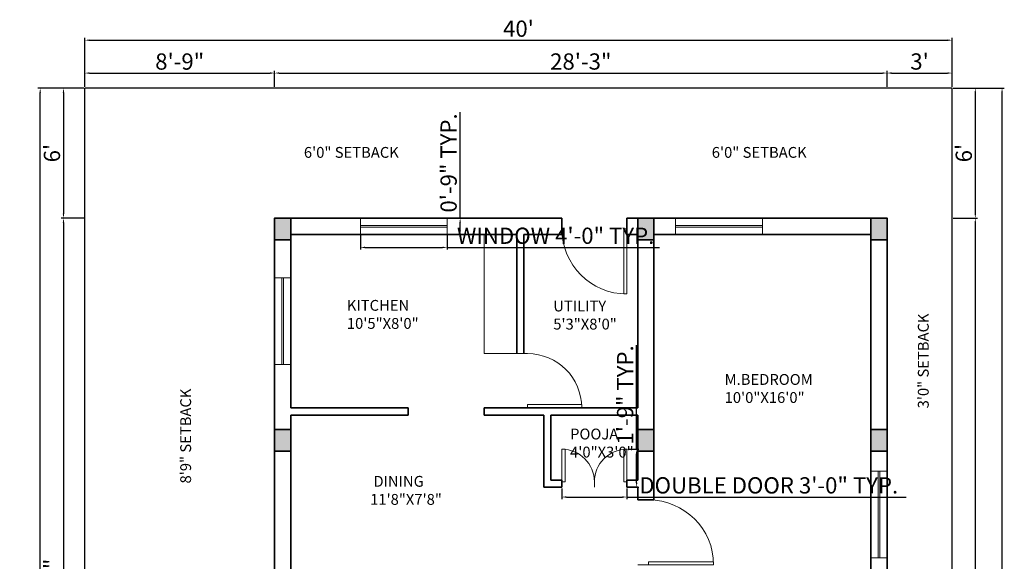
# Model space of a CAD drawing. Units: inches. Extents: x 3321 to 5237, y 11 to 1752.
# Tile 2 of 43: x 3321 to 3866, y 529 to 828. Entities that reach past the tile are written whole.
import ezdxf

# ---------------------------------------------------------------- set-up
doc = ezdxf.new("R2010")
doc.units = ezdxf.units.IN
for name, color, linetype, lineweight in [('A-ANNO-DIMS', 2, 'Continuous', 18), ('A-ANNO-TEXT', 7, 'Continuous', 18), ('A-AREA-IDEN', 7, 'Continuous', 18), ('A-COLS', 1, 'Continuous', 35), ('A-DOOR', 4, 'Continuous', 18), ('A-FLOR-CASE', 8, 'Continuous', 18), ('A-GLAZ', 5, 'Continuous', 18), ('A-WALL', 7, 'Continuous', 35), ('C-PROP', 7, 'Continuous', 30)]:
    doc.layers.add(name, color=color, linetype=linetype, lineweight=lineweight)
doc.styles.get("Standard").update_dxf_attribs({"font": 'arial.ttf'})
doc.dimstyles.new('ISO-25', dxfattribs={"dimtxt": 9, "dimasz": 2.5, "dimexe": 1.25, "dimexo": 0.625, "dimtad": 1, "dimdec": 1, "dimlunit": 3, "dimtxsty": 'Standard', "dimcen": 2.5, "dimclrd": 4, "dimclre": 4, "dimclrt": 256, "dimadec": 0, "dimazin": 0, "dimtfac": 1, "dimtdec": 1, "dimtmove": 0, "dimatfit": 3, "dimfxl": 1, "dimarcsym": 0})

# ---------------------------------------------------------------- blocks, each defined once
blk = doc.blocks.new('*U4')
for p, q in [((0, 0), (0, -6)), ((-36, 0), (-36, -6))]:
    blk.add_line(p, q)
blk.add_lwpolyline([(0, 0), (0, 36), (-1.75, 36), (-1.75, 0)], close=True)
blk.add_arc((0, 0), 36, 90, 180)
blk = doc.blocks.new('*U5')
for p, q in [((0, 0), (0, -6)), ((-30, 0), (-30, -6))]:
    blk.add_line(p, q)
blk.add_lwpolyline([(0, 0), (0, 30), (-1.75, 30), (-1.75, 0)], close=True)
blk.add_arc((0, 0), 30, 90, 180)
blk = doc.blocks.new('*U11')
for p, q in [((0, 0), (0, -6)), ((36, 0), (36, -6))]:
    blk.add_line(p, q)
blk.add_lwpolyline([(0, 0), (0, 36), (1.75, 36), (1.75, 0)], close=True)
blk.add_arc((0, 0), 36, 0, 90)
blk = doc.blocks.new('*D79')
at = {"layer": 'A-ANNO-DIMS', "color": 0, "lineweight": -2, "transparency": 16777216}
for p, q in [((3356.06, 790.61), (3343.59, 790.61)), ((3344.84, 788.11), (3344.84, 721.11)), ((3356.06, 718.61), (3343.59, 718.61))]:
    blk.add_line(p, q, dxfattribs=at)
at = {"layer": 'A-ANNO-DIMS', "color": 0, "transparency": 16777216}
for points in [[(3344.42, 788.11), (3345.26, 788.11), (3344.84, 790.61)], [(3344.42, 721.11), (3345.26, 721.11), (3344.84, 718.61)]]:
    blk.add_solid(points, dxfattribs=at)
at = {"layer": 'Defpoints', "color": 0, "transparency": 16777216}
for p in [(3356.69, 790.61), (3344.84, 718.61), (3356.69, 718.61)]:
    blk.add_point(p, dxfattribs=at)
at = {"layer": 'A-ANNO-DIMS', "color": 0, "transparency": 16777216, "insert": (3339.62, 754.61), "char_height": 9, "attachment_point": 5, "rotation": 90}
blk.add_mtext("6'", dxfattribs=at)
blk = doc.blocks.new('*D70')
at = {"layer": 'A-ANNO-DIMS', "color": 0, "lineweight": -2, "transparency": 16777216}
for p, q in [((3356.06, 718.61), (3343.59, 718.61)), ((3344.84, 716.11), (3344.84, 310.11)), ((3356.06, 307.61), (3343.59, 307.61))]:
    blk.add_line(p, q, dxfattribs=at)
at = {"layer": 'A-ANNO-DIMS', "color": 0, "transparency": 16777216}
for points in [[(3344.42, 716.11), (3345.26, 716.11), (3344.84, 718.61)], [(3344.42, 310.11), (3345.26, 310.11), (3344.84, 307.61)]]:
    blk.add_solid(points, dxfattribs=at)
at = {"layer": 'Defpoints', "color": 0, "transparency": 16777216}
for p in [(3356.69, 718.61), (3344.84, 307.61), (3356.69, 307.61)]:
    blk.add_point(p, dxfattribs=at)
at = {"layer": 'A-ANNO-DIMS', "color": 0, "transparency": 16777216, "insert": (3339.62, 513.11), "char_height": 9, "attachment_point": 5, "rotation": 90}
blk.add_mtext('34\'-3"', dxfattribs=at)
blk = doc.blocks.new('*D71')
at = {"layer": 'A-ANNO-DIMS', "color": 0, "lineweight": -2, "transparency": 16777216}
for p, q in [((3356.69, 791.23), (3356.69, 800.18)), ((3359.19, 798.93), (3459.19, 798.93)), ((3461.69, 791.23), (3461.69, 800.18))]:
    blk.add_line(p, q, dxfattribs=at)
at = {"layer": 'A-ANNO-DIMS', "color": 0, "transparency": 16777216}
for points in [[(3359.19, 799.35), (3359.19, 798.52), (3356.69, 798.93)], [(3459.19, 799.35), (3459.19, 798.52), (3461.69, 798.93)]]:
    blk.add_solid(points, dxfattribs=at)
at = {"layer": 'Defpoints', "color": 0, "transparency": 16777216}
for p in [(3461.69, 798.93), (3356.69, 790.61), (3461.69, 790.61)]:
    blk.add_point(p, dxfattribs=at)
at = {"layer": 'A-ANNO-DIMS', "color": 0, "transparency": 16777216, "insert": (3409.19, 804.15), "char_height": 9, "attachment_point": 5}
blk.add_mtext('8\'-9"', dxfattribs=at)
blk = doc.blocks.new('*D72')
at = {"layer": 'A-ANNO-DIMS', "color": 0, "lineweight": -2, "transparency": 16777216}
for p, q in [((3461.69, 791.23), (3461.69, 800.18)), ((3464.19, 798.93), (3798.19, 798.93)), ((3800.69, 791.23), (3800.69, 800.18))]:
    blk.add_line(p, q, dxfattribs=at)
at = {"layer": 'A-ANNO-DIMS', "color": 0, "transparency": 16777216}
for points in [[(3464.19, 799.35), (3464.19, 798.52), (3461.69, 798.93)], [(3798.19, 799.35), (3798.19, 798.52), (3800.69, 798.93)]]:
    blk.add_solid(points, dxfattribs=at)
at = {"layer": 'Defpoints', "color": 0, "transparency": 16777216}
for p in [(3800.69, 798.93), (3461.69, 790.61), (3800.69, 790.61)]:
    blk.add_point(p, dxfattribs=at)
at = {"layer": 'A-ANNO-DIMS', "color": 0, "transparency": 16777216, "insert": (3631.19, 804.16), "char_height": 9, "attachment_point": 5}
blk.add_mtext('28\'-3"', dxfattribs=at)
blk = doc.blocks.new('*D81')
at = {"layer": 'A-ANNO-DIMS', "color": 0, "lineweight": -2, "transparency": 16777216}
for p, q in [((3800.69, 791.23), (3800.69, 800.18)), ((3803.19, 798.93), (3834.19, 798.93)), ((3836.69, 791.23), (3836.69, 800.18))]:
    blk.add_line(p, q, dxfattribs=at)
at = {"layer": 'A-ANNO-DIMS', "color": 0, "transparency": 16777216}
for points in [[(3803.19, 799.35), (3803.19, 798.52), (3800.69, 798.93)], [(3834.19, 799.35), (3834.19, 798.52), (3836.69, 798.93)]]:
    blk.add_solid(points, dxfattribs=at)
at = {"layer": 'Defpoints', "color": 0, "transparency": 16777216}
for p in [(3836.69, 798.93), (3800.69, 790.61), (3836.69, 790.61)]:
    blk.add_point(p, dxfattribs=at)
at = {"layer": 'A-ANNO-DIMS', "color": 0, "transparency": 16777216, "insert": (3818.69, 804.16), "char_height": 9, "attachment_point": 5}
blk.add_mtext("3'", dxfattribs=at)
blk = doc.blocks.new('*D73')
at = {"layer": 'A-ANNO-DIMS', "color": 0, "lineweight": -2, "transparency": 16777216}
for p, q in [((3837.31, 790.61), (3850.8, 790.61)), ((3849.55, 788.11), (3849.55, 721.11)), ((3837.31, 718.61), (3850.8, 718.61))]:
    blk.add_line(p, q, dxfattribs=at)
at = {"layer": 'A-ANNO-DIMS', "color": 0, "transparency": 16777216}
for points in [[(3849.13, 788.11), (3849.96, 788.11), (3849.55, 790.61)], [(3849.13, 721.11), (3849.96, 721.11), (3849.55, 718.61)]]:
    blk.add_solid(points, dxfattribs=at)
at = {"layer": 'Defpoints', "color": 0, "transparency": 16777216}
for p in [(3836.69, 790.61), (3836.69, 718.61), (3849.55, 718.61)]:
    blk.add_point(p, dxfattribs=at)
at = {"layer": 'A-ANNO-DIMS', "color": 0, "transparency": 16777216, "insert": (3844.33, 754.61), "char_height": 9, "attachment_point": 5, "rotation": 90}
blk.add_mtext("6'", dxfattribs=at)
blk = doc.blocks.new('*D74')
at = {"layer": 'A-ANNO-DIMS', "color": 0, "lineweight": -2, "transparency": 16777216}
for p, q in [((3837.31, 718.61), (3850.8, 718.61)), ((3849.55, 716.11), (3849.55, 177.11)), ((3837.31, 174.61), (3850.8, 174.61))]:
    blk.add_line(p, q, dxfattribs=at)
at = {"layer": 'A-ANNO-DIMS', "color": 0, "transparency": 16777216}
for points in [[(3849.13, 716.11), (3849.96, 716.11), (3849.55, 718.61)], [(3849.13, 177.11), (3849.96, 177.11), (3849.55, 174.61)]]:
    blk.add_solid(points, dxfattribs=at)
at = {"layer": 'Defpoints', "color": 0, "transparency": 16777216}
for p in [(3836.69, 718.61), (3836.69, 174.61), (3849.55, 174.61)]:
    blk.add_point(p, dxfattribs=at)
at = {"layer": 'A-ANNO-DIMS', "color": 0, "transparency": 16777216, "insert": (3844.35, 446.61), "char_height": 9, "attachment_point": 5, "rotation": 90}
blk.add_mtext('45\'-4"', dxfattribs=at)
blk = doc.blocks.new('*D82')
at = {"layer": 'A-ANNO-DIMS', "color": 0, "lineweight": -2, "transparency": 16777216}
for p, q in [((3356.69, 791.23), (3356.69, 818.38)), ((3836.69, 791.23), (3836.69, 818.38)), ((3359.19, 817.13), (3834.19, 817.13))]:
    blk.add_line(p, q, dxfattribs=at)
at = {"layer": 'A-ANNO-DIMS', "color": 0, "transparency": 16777216}
for points in [[(3359.19, 817.55), (3359.19, 816.72), (3356.69, 817.13)], [(3834.19, 817.55), (3834.19, 816.72), (3836.69, 817.13)]]:
    blk.add_solid(points, dxfattribs=at)
at = {"layer": 'Defpoints', "color": 0, "transparency": 16777216}
for p in [(3836.69, 817.13), (3356.69, 790.61), (3836.69, 790.61)]:
    blk.add_point(p, dxfattribs=at)
at = {"layer": 'A-ANNO-DIMS', "color": 0, "transparency": 16777216, "insert": (3596.69, 822.35), "char_height": 9, "attachment_point": 5}
blk.add_mtext("40'", dxfattribs=at)
blk = doc.blocks.new('*D83')
at = {"layer": 'A-ANNO-DIMS', "color": 0, "lineweight": -2, "transparency": 16777216}
for p, q in [((3356.06, 790.61), (3330.71, 790.61)), ((3331.96, 73.11), (3331.96, 788.11)), ((3356.06, 70.61), (3330.71, 70.61))]:
    blk.add_line(p, q, dxfattribs=at)
at = {"layer": 'A-ANNO-DIMS', "color": 0, "transparency": 16777216}
for points in [[(3331.55, 788.11), (3332.38, 788.11), (3331.96, 790.61)], [(3331.55, 73.11), (3332.38, 73.11), (3331.96, 70.61)]]:
    blk.add_solid(points, dxfattribs=at)
at = {"layer": 'Defpoints', "color": 0, "transparency": 16777216}
for p in [(3331.96, 790.61), (3356.69, 790.61), (3356.69, 70.61)]:
    blk.add_point(p, dxfattribs=at)
at = {"layer": 'A-ANNO-DIMS', "color": 0, "transparency": 16777216, "insert": (3326.74, 430.61), "char_height": 9, "attachment_point": 5, "rotation": 90}
blk.add_mtext("60'", dxfattribs=at)
blk = doc.blocks.new('*D85')
at = {"layer": 'A-ANNO-DIMS', "color": 0, "lineweight": -2, "transparency": 16777216}
for p, q in [((3837.31, 790.61), (3865.6, 790.61)), ((3864.35, 73.11), (3864.35, 788.11)), ((3837.31, 70.61), (3865.6, 70.61))]:
    blk.add_line(p, q, dxfattribs=at)
at = {"layer": 'A-ANNO-DIMS', "color": 0, "transparency": 16777216}
for points in [[(3863.93, 788.11), (3864.76, 788.11), (3864.35, 790.61)], [(3863.93, 73.11), (3864.76, 73.11), (3864.35, 70.61)]]:
    blk.add_solid(points, dxfattribs=at)
at = {"layer": 'Defpoints', "color": 0, "transparency": 16777216}
for p in [(3836.69, 790.61), (3864.35, 790.61), (3836.69, 70.61)]:
    blk.add_point(p, dxfattribs=at)
at = {"layer": 'A-ANNO-DIMS', "color": 0, "transparency": 16777216, "insert": (3859.13, 430.61), "char_height": 9, "attachment_point": 5, "rotation": 90}
blk.add_mtext("60'", dxfattribs=at)
blk = doc.blocks.new('COL-9X12-BASE-PLAN')
h = blk.add_hatch(color=256)
h.dxf.hatch_style = 1
h.paths.add_polyline_path([(0, 0), (9, 0), (9, 12), (0, 12)])
blk.add_lwpolyline([(0, 0), (9, 0), (9, 12), (0, 12)], close=True)
blk = doc.blocks.new('WIN-48IN-9IN-WALL')
for p, q in [((0, 0), (0, 9)), ((48, 0), (48, 9)), ((0, 5), (48, 5)), ((0, 4), (48, 4))]:
    blk.add_line(p, q)
blk = doc.blocks.new('DOOR-DOUBLE-36IN')
for p, q in [((0, 3), (0, 0)), ((18, 3), (18, 0)), ((18, 3), (18, 0)), ((36, 3), (36, 0))]:
    blk.add_line(p, q)
for points in [[(0, 3), (0, 21), (1.75, 21), (1.75, 3)], [(36, 3), (36, 21), (34.25, 21), (34.25, 3)]]:
    blk.add_lwpolyline(points, close=True)
for centre, start, end in [((0, 3), 0, 90), ((36, 3), 90, 180)]:
    blk.add_arc(centre, 18, start, end)
blk = doc.blocks.new('PROPERTY-40X60FT')
for p, q in [((0, 720), (480, 720)), ((0, 720), (0, 0)), ((480, 720), (480, 0)), ((0, 0), (480, 0))]:
    blk.add_line(p, q)
blk = doc.blocks.new('*D165')
at = {"layer": 'A-ANNO-DIMS', "color": 4, "lineweight": -2, "transparency": 16777216}
for p, q in [((3509.19, 708.98), (3509.19, 701.16)), ((3557.19, 708.98), (3557.19, 701.16)), ((3511.69, 702.41), (3554.69, 702.41)), ((3557.19, 702.41), (3674.83, 702.41))]:
    blk.add_line(p, q, dxfattribs=at)
at = {"layer": 'A-ANNO-DIMS', "color": 4, "transparency": 16777216}
for points in [[(3511.69, 702.82), (3511.69, 701.99), (3509.19, 702.41)], [(3554.69, 702.82), (3554.69, 701.99), (3557.19, 702.41)]]:
    blk.add_solid(points, dxfattribs=at)
at = {"layer": 'Defpoints', "color": 0, "transparency": 16777216}
for p in [(3509.19, 709.61), (3557.19, 709.61), (3557.19, 702.41)]:
    blk.add_point(p, dxfattribs=at)
at = {"layer": 'A-ANNO-DIMS', "transparency": 16777216, "insert": (3617.26, 707.69), "char_height": 9, "attachment_point": 5}
blk.add_mtext('WINDOW 4\'-0" TYP.', dxfattribs=at)
blk = doc.blocks.new('*D166')
at = {"layer": 'A-ANNO-DIMS', "color": 4, "lineweight": -2, "transparency": 16777216}
for p, q in [((3564.39, 718.61), (3564.39, 777.22)), ((3557.81, 718.61), (3565.64, 718.61)), ((3564.39, 712.11), (3564.39, 716.11)), ((3557.81, 709.61), (3565.64, 709.61))]:
    blk.add_line(p, q, dxfattribs=at)
at = {"layer": 'A-ANNO-DIMS', "color": 4, "transparency": 16777216}
for points in [[(3563.97, 716.11), (3564.81, 716.11), (3564.39, 718.61)], [(3563.97, 712.11), (3564.81, 712.11), (3564.39, 709.61)]]:
    blk.add_solid(points, dxfattribs=at)
at = {"layer": 'Defpoints', "color": 0, "transparency": 16777216}
for p in [(3557.19, 718.61), (3564.39, 718.61), (3557.19, 709.61)]:
    blk.add_point(p, dxfattribs=at)
at = {"layer": 'A-ANNO-DIMS', "transparency": 16777216, "insert": (3559.17, 749.16), "char_height": 9, "attachment_point": 5, "rotation": 90}
blk.add_mtext('0\'-9" TYP.', dxfattribs=at)
blk = doc.blocks.new('*D173')
at = {"layer": 'A-ANNO-DIMS', "color": 4, "lineweight": -2, "transparency": 16777216}
for p, q in [((3620.69, 568.98), (3620.69, 562.96)), ((3656.69, 568.98), (3656.69, 562.96)), ((3623.19, 564.21), (3654.19, 564.21)), ((3656.69, 564.21), (3811.26, 564.21))]:
    blk.add_line(p, q, dxfattribs=at)
at = {"layer": 'A-ANNO-DIMS', "color": 4, "transparency": 16777216}
for points in [[(3623.19, 564.62), (3623.19, 563.79), (3620.69, 564.21)], [(3654.19, 564.62), (3654.19, 563.79), (3656.69, 564.21)]]:
    blk.add_solid(points, dxfattribs=at)
at = {"layer": 'Defpoints', "color": 0, "transparency": 16777216}
for p in [(3620.69, 569.61), (3656.69, 569.61), (3656.69, 564.21)]:
    blk.add_point(p, dxfattribs=at)
at = {"layer": 'A-ANNO-DIMS', "transparency": 16777216, "insert": (3735.22, 569.49), "char_height": 9, "attachment_point": 5}
blk.add_mtext('DOUBLE DOOR 3\'-0" TYP.', dxfattribs=at)
blk = doc.blocks.new('*D174')
at = {"layer": 'A-ANNO-DIMS', "color": 4, "lineweight": -2, "transparency": 16777216}
for p, q in [((3662.09, 590.61), (3662.09, 648.37)), ((3657.31, 590.61), (3663.34, 590.61)), ((3662.09, 572.11), (3662.09, 588.11)), ((3657.31, 569.61), (3663.34, 569.61))]:
    blk.add_line(p, q, dxfattribs=at)
at = {"layer": 'A-ANNO-DIMS', "color": 4, "transparency": 16777216}
for points in [[(3661.67, 588.11), (3662.51, 588.11), (3662.09, 590.61)], [(3661.67, 572.11), (3662.51, 572.11), (3662.09, 569.61)]]:
    blk.add_solid(points, dxfattribs=at)
at = {"layer": 'Defpoints', "color": 0, "transparency": 16777216}
for p in [(3656.69, 590.61), (3662.09, 590.61), (3656.69, 569.61)]:
    blk.add_point(p, dxfattribs=at)
at = {"layer": 'A-ANNO-DIMS', "transparency": 16777216, "insert": (3656.87, 620.74), "char_height": 9, "attachment_point": 5, "rotation": 90}
blk.add_mtext('1\'-9" TYP.', dxfattribs=at)

msp = doc.modelspace()

# ---------------------------------------------------------------- linework, layer by layer
at = {"layer": 'A-FLOR-CASE'}
for p, q in [((3577.69, 709.61), (3577.69, 643.61)), ((3577.69, 643.61), (3599.69, 643.61))]:
    msp.add_line(p, q, dxfattribs=at)
at = {"layer": 'A-WALL'}
for p, q in [((3461.69, 718.61), (3461.69, 307.61)), ((3461.69, 718.61), (3620.69, 718.61)), ((3620.69, 718.61), (3620.69, 709.61)), ((3656.69, 718.61), (3656.69, 709.61)), ((3656.69, 718.61), (3800.69, 718.61)), ((3800.69, 718.61), (3800.69, 174.61)), ((3470.69, 709.61), (3470.69, 613.61)), ((3470.69, 709.61), (3595.69, 709.61)), ((3595.69, 709.61), (3595.69, 643.61)), ((3599.69, 709.61), (3599.69, 643.61)), ((3599.69, 709.61), (3620.69, 709.61)), ((3656.69, 709.61), (3662.69, 709.61)), ((3662.69, 709.61), (3662.69, 613.61)), ((3671.69, 709.61), (3671.69, 562.61)), ((3671.69, 709.61), (3791.69, 709.61)), ((3791.69, 709.61), (3791.69, 517.61)), ((3470.69, 613.61), (3535.69, 613.61)), ((3535.69, 613.61), (3535.69, 609.61)), ((3577.69, 613.61), (3577.69, 609.61)), ((3577.69, 613.61), (3662.69, 613.61)), ((3470.69, 609.61), (3470.69, 517.61)), ((3470.69, 609.61), (3535.69, 609.61)), ((3577.69, 609.61), (3610.69, 609.61)), ((3610.69, 609.61), (3610.69, 569.61)), ((3614.69, 609.61), (3614.69, 573.61)), ((3614.69, 609.61), (3662.69, 609.61)), ((3662.69, 609.61), (3662.69, 573.61)), ((3614.69, 573.61), (3620.69, 573.61)), ((3620.69, 573.61), (3620.69, 569.61)), ((3656.69, 573.61), (3662.69, 573.61)), ((3656.69, 573.61), (3656.69, 569.61)), ((3610.69, 569.61), (3620.69, 569.61)), ((3656.69, 569.61), (3662.69, 569.61)), ((3662.69, 569.61), (3662.69, 562.61)), ((3662.69, 562.61), (3671.69, 562.61))]:
    msp.add_line(p, q, dxfattribs=at)

# ---------------------------------------------------------------- block references
at = {"layer": 'A-COLS'}
for p in [(3461.69, 706.61), (3662.69, 706.61), (3791.69, 706.61), (3461.69, 589.61), (3662.69, 589.61), (3791.69, 589.61)]:
    msp.add_blockref('COL-9X12-BASE-PLAN', p, dxfattribs=at)
at = {"layer": 'A-DOOR'}
for name, p, rotation in [('*U11', (3656.69, 712.61), 180), ('*U5', (3601.69, 613.61), 270), ('*U4', (3668.69, 526.61), 270)]:
    msp.add_blockref(name, p, dxfattribs=dict(at, rotation=rotation))
msp.add_blockref('DOOR-DOUBLE-36IN', (3620.69, 569.61), dxfattribs=at)
at = {"layer": 'A-GLAZ'}
for p in [(3509.19, 709.61), (3683.69, 709.61)]:
    msp.add_blockref('WIN-48IN-9IN-WALL', p, dxfattribs=at)
for p, rotation in [((3470.69, 637.61), 89.99999999999925), ((3800.69, 530.61), 89.9999999999993)]:
    msp.add_blockref('WIN-48IN-9IN-WALL', p, dxfattribs=dict(at, rotation=rotation))
at = {"layer": 'C-PROP', "rotation": 180}
msp.add_blockref('PROPERTY-40X60FT', (3836.69, 790.61), dxfattribs=at)

# ---------------------------------------------------------------- texts
at = {"layer": 'A-ANNO-TEXT', "char_height": 6, "attachment_point": 1}
for insert in [(3477.92, 758.01), (3703.67, 758.01)]:
    msp.add_mtext_dynamic_manual_height_columns('6\'0" SETBACK', width=97.3114, gutter_width=25, heights=[0], dxfattribs=dict(at, insert=insert))
at = {"layer": 'A-ANNO-TEXT', "char_height": 6, "attachment_point": 1, "rotation": 90}
for s, insert in [('3\'0" SETBACK', (3817.76, 613.28)), ('8\'9" SETBACK', (3409.48, 571.69))]:
    msp.add_mtext_dynamic_manual_height_columns(s, width=97.3114, gutter_width=25, heights=[0], dxfattribs=dict(at, insert=insert))
at = {"layer": 'A-AREA-IDEN', "char_height": 6, "attachment_point": 1}
for s, insert in [('KITCHEN\\P10\'5"X8\'0"', (3501.7, 673.32)), ('UTILITY\\P5\'3"X8\'0"', (3615.93, 672.95)), ('M.BEDROOM\\P10\'0"X16\'0"', (3710.8, 632.3)), ('POOJA\\P4\'0"X3\'0"', (3625.25, 602.08)), (' DINING\\P11\'8"X7\'8"', (3514.57, 575.89))]:
    msp.add_mtext_dynamic_manual_height_columns(s, width=97.3114, gutter_width=25, heights=[0], dxfattribs=dict(at, insert=insert))

# ---------------------------------------------------------------- dimensions: what is measured, and where the dimension line sits
at = {"layer": 'A-ANNO-DIMS'}
for base, p1, p2, override, picture, middle in [((3836.69, 817.13), (3356.69, 790.61), (3836.69, 790.61), {"dimclrd": 0, "dimclre": 0, "dimclrt": 0}, '*D82', (3596.69, 822.35)), ((3461.69, 798.93), (3356.69, 790.61), (3461.69, 790.61), {"dimclrd": 0, "dimclre": 0, "dimclrt": 0}, '*D71', (3409.19, 804.15)), ((3800.69, 798.93), (3461.69, 790.61), (3800.69, 790.61), {"dimclrd": 0, "dimclre": 0, "dimclrt": 0, "dimtmove": 1}, '*D72', (3631.19, 804.16)), ((3836.69, 798.93), (3800.69, 790.61), (3836.69, 790.61), {"dimclrd": 0, "dimclre": 0, "dimclrt": 0, "dimtmove": 1}, '*D81', (3818.69, 804.16))]:
    dim = msp.add_linear_dim(base=base, p1=p1, p2=p2, dimstyle='ISO-25', override=override, dxfattribs=at)
    dim.commit()
    dim.dimension.update_dxf_attribs({"geometry": picture, "text_midpoint": middle})
for base, p1, p2, angle, override, picture, middle in [((3331.96, 790.61), (3356.69, 70.61), (3356.69, 790.61), 270, {"dimclrd": 0, "dimclre": 0, "dimclrt": 0}, '*D83', (3326.74, 430.61)), ((3344.84, 718.61), (3356.69, 790.61), (3356.69, 718.61), 90, {"dimclrd": 0, "dimclre": 0, "dimclrt": 0}, '*D79', (3339.62, 754.61)), ((3849.55, 718.61), (3836.69, 790.61), (3836.69, 718.61), 90, {"dimclrd": 0, "dimclre": 0, "dimclrt": 0}, '*D73', (3844.33, 754.61)), ((3864.35, 790.61), (3836.69, 70.61), (3836.69, 790.61), 270, {"dimclrd": 0, "dimclre": 0, "dimclrt": 0}, '*D85', (3859.13, 430.61)), ((3344.84, 307.61), (3356.69, 718.61), (3356.69, 307.61), 90, {"dimclrd": 0, "dimclre": 0, "dimclrt": 0, "dimtmove": 1}, '*D70', (3339.62, 513.11)), ((3849.55, 174.61), (3836.69, 718.61), (3836.69, 174.61), 90, {"dimclrd": 0, "dimclre": 0, "dimclrt": 0, "dimtmove": 1}, '*D74', (3844.35, 446.61))]:
    dim = msp.add_linear_dim(base=base, p1=p1, p2=p2, angle=angle, dimstyle='ISO-25', override=override, dxfattribs=at)
    dim.commit()
    dim.dimension.update_dxf_attribs({"geometry": picture, "text_midpoint": middle})
for base, p1, p2, picture, middle in [((3564.39, 718.61), (3557.19, 709.61), (3557.19, 718.61), '*D166', (3559.17, 749.16)), ((3662.09, 590.61), (3656.69, 569.61), (3656.69, 590.61), '*D174', (3656.87, 620.74))]:
    dim = msp.add_linear_dim(base=base, p1=p1, p2=p2, angle=90, text='<> TYP.', dimstyle='ISO-25', override={"dimdec": 1, "dimlfac": 1, "dimrnd": 0, "dimzin": 1, "dimdsep": 46, "dimlunit": 4, "dimfrac": 2}, dxfattribs=at)
    dim.commit()
    dim.dimension.update_dxf_attribs({"geometry": picture, "text_midpoint": middle})
for base, p1, p2, text, picture, middle in [((3557.19, 702.41), (3509.19, 709.61), (3557.19, 709.61), 'WINDOW <> TYP.', '*D165', (3617.26, 707.69)), ((3656.69, 564.21), (3620.69, 569.61), (3656.69, 569.61), 'DOUBLE DOOR <> TYP.', '*D173', (3735.22, 569.49))]:
    dim = msp.add_linear_dim(base=base, p1=p1, p2=p2, text=text, dimstyle='ISO-25', override={"dimdec": 1, "dimlfac": 1, "dimrnd": 0, "dimzin": 1, "dimdsep": 46, "dimlunit": 4, "dimfrac": 2}, dxfattribs=at)
    dim.commit()
    dim.dimension.update_dxf_attribs({"geometry": picture, "text_midpoint": middle})

doc.saveas('drawing.dxf')
